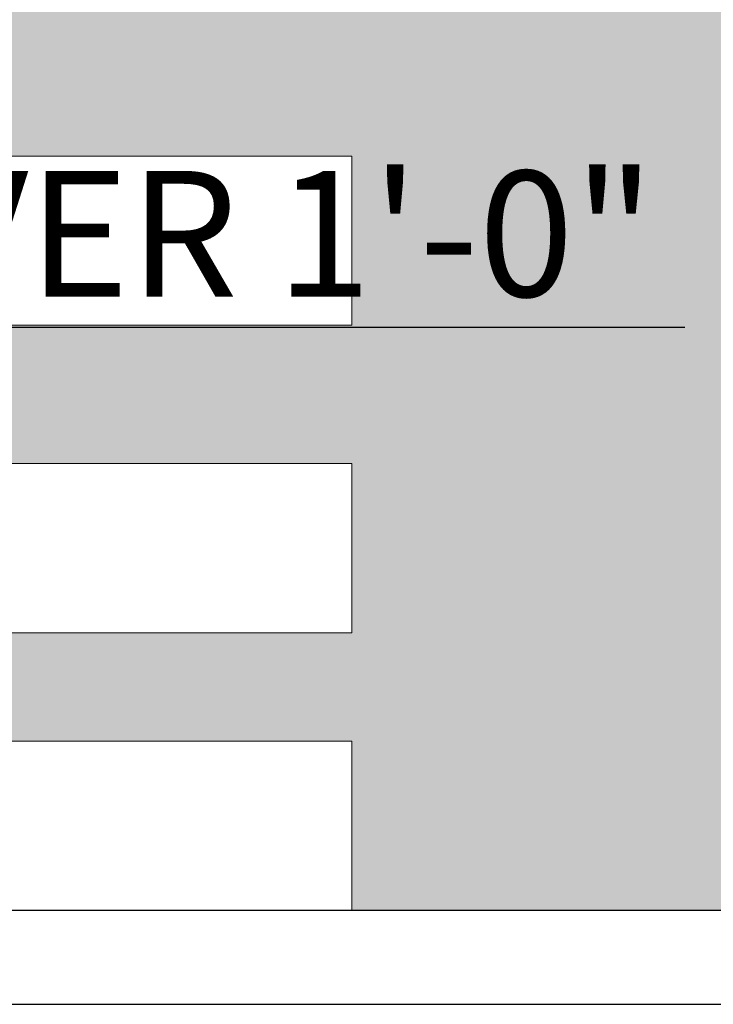
# Model space of a CAD drawing. Units: inches. Extents: x 459864 to 460310, y 324185 to 324787.
# Tile 43 of 112: x 460094 to 460127, y 324195 to 324242. Entities that reach past the tile are written whole.
import ezdxf

# ---------------------------------------------------------------- set-up
doc = ezdxf.new("R2010")
doc.units = ezdxf.units.IN
for name, color, linetype, lineweight in [('A-ANNO-DIMS', 2, 'Continuous', 18), ('C-PROP', 7, 'Continuous', 30), ('L-HRDS', 9, 'Continuous', 18), ('L-SITE-PATT', 252, 'Continuous', 13)]:
    doc.layers.add(name, color=color, linetype=linetype, lineweight=lineweight)
doc.styles.get("Standard").update_dxf_attribs({"font": 'arial.ttf'})
doc.dimstyles.new('ISO-25', dxfattribs={"dimtxt": 6, "dimasz": 2.5, "dimexe": 1.25, "dimexo": 0.625, "dimtad": 1, "dimdec": 1, "dimlunit": 3, "dimtxsty": 'Standard', "dimcen": 2.5, "dimadec": 0, "dimazin": 0, "dimtfac": 1, "dimtdec": 1, "dimtmove": 0, "dimatfit": 3, "dimfxl": 1, "dimarcsym": 0})

# ---------------------------------------------------------------- blocks, each defined once
blk = doc.blocks.new('*D28')
at = {"layer": 'A-ANNO-DIMS', "color": 0, "lineweight": -2, "transparency": 16777216}
for p, q in [((460148.65, 324370.7), (460136.025, 324370.7)), ((460137.275, 324368.2), (460137.275, 324293.2)), ((460148.65, 324290.7), (460136.025, 324290.7)), ((460137.275, 324290.7), (460137.275, 324198.69))]:
    blk.add_line(p, q, dxfattribs=at)
at = {"layer": 'A-ANNO-DIMS', "color": 0, "transparency": 16777216}
for points in [[(460136.858, 324368.2), (460137.692, 324368.2), (460137.275, 324370.7)], [(460136.858, 324293.2), (460137.692, 324293.2), (460137.275, 324290.7)]]:
    blk.add_solid(points, dxfattribs=at)
at = {"layer": 'Defpoints', "color": 0, "transparency": 16777216}
for p in [(460149.275, 324370.7), (460137.275, 324290.7), (460149.275, 324290.7)]:
    blk.add_point(p, dxfattribs=at)
at = {"layer": 'A-ANNO-DIMS', "color": 0, "transparency": 16777216, "insert": (460133.363, 324243.445), "char_height": 6, "attachment_point": 5, "rotation": 90}
blk.add_mtext('QUEEN BED 6\'-8" TYP.', dxfattribs=at)
blk = doc.blocks.new('*D36')
at = {"layer": 'A-ANNO-DIMS', "color": 0, "lineweight": -2, "transparency": 16777216}
for p, q in [((460063.861, 324228.483), (460063.861, 324226.056)), ((460075.876, 324228.483), (460075.876, 324226.056)), ((460066.361, 324227.306), (460073.376, 324227.306)), ((460075.876, 324227.306), (460126.021, 324227.306))]:
    blk.add_line(p, q, dxfattribs=at)
at = {"layer": 'A-ANNO-DIMS', "color": 0, "transparency": 16777216}
for points in [[(460066.361, 324227.722), (460066.361, 324226.889), (460063.861, 324227.306)], [(460073.376, 324227.722), (460073.376, 324226.889), (460075.876, 324227.306)]]:
    blk.add_solid(points, dxfattribs=at)
at = {"layer": 'Defpoints', "color": 0, "transparency": 16777216}
for p in [(460063.861, 324229.108), (460075.876, 324229.108), (460075.876, 324227.306)]:
    blk.add_point(p, dxfattribs=at)
at = {"layer": 'A-ANNO-DIMS', "color": 0, "transparency": 16777216, "insert": (460102.199, 324230.994), "char_height": 6, "attachment_point": 5}
blk.add_mtext('PAVER 1\'-0"', dxfattribs=at)

msp = doc.modelspace()

# ---------------------------------------------------------------- hatches: boundary and pattern name
at = {"layer": 'L-SITE-PATT'}
h = msp.add_hatch(dxfattribs=at)
h.set_pattern_fill('DOTS', color=256)
h.paths.add_polyline_path([(460269.804, 324283.483), (460247.115, 324283.483), (460121.929, 324283.483), (460121.929, 324252.473), (460117.429, 324252.473), (460110.124, 324252.473), (460110.124, 324243.287), (460080.83, 324243.287), (460080.83, 324252.473), (460061.115, 324252.473), (460061.115, 324251.882), (460077.909, 324251.882), (460077.909, 324199.483), (460080.83, 324199.483), (460080.83, 324207.553), (460110.124, 324207.553), (460110.124, 324199.483), (460110.813, 324199.483), (460262.115, 324199.483), (460269.804, 324199.483)], flags=17)
edge = h.paths.add_edge_path(flags=0)
edge.add_ellipse((460222.59, 324263.813), major_axis=(-8.485, 8.485), ratio=1, start_angle=405, end_angle=495, ccw=False)
edge.add_line((460214.821, 324254.66), (460214.832, 324254.666))
edge.add_ellipse((460222.59, 324263.813), major_axis=(-8.485, 8.485), ratio=1, start_angle=405, end_angle=495, ccw=False)
edge.add_line((460210.759, 324261.781), (460210.768, 324261.787))
edge.add_ellipse((460222.59, 324263.813), major_axis=(-8.485, 8.485), ratio=1, start_angle=405, end_angle=495, ccw=False)
edge.add_ellipse((460222.59, 324263.813), major_axis=(-8.485, 8.485), ratio=1, start_angle=392.754, end_angle=405, ccw=False)
edge.add_ellipse((460222.59, 324263.813), major_axis=(-8.485, 8.485), ratio=1, start_angle=380.9347, end_angle=392.754, ccw=False)
edge.add_line((460211.337, 324267.985), (460211.34, 324267.985))
edge.add_ellipse((460222.59, 324263.813), major_axis=(-8.485, 8.485), ratio=1, start_angle=380.9347, end_angle=392.754, ccw=False)
edge.add_ellipse((460222.59, 324263.813), major_axis=(-8.485, 8.485), ratio=1, start_angle=347.9015, end_angle=380.9347, ccw=False)
edge.add_ellipse((460222.59, 324263.813), major_axis=(-8.485, 8.485), ratio=1, start_angle=327.0619, end_angle=347.9015, ccw=False)
edge.add_ellipse((460222.59, 324263.813), major_axis=(-8.485, 8.485), ratio=1, start_angle=278.3246, end_angle=327.0619, ccw=False)
edge.add_line((460225.158, 324275.536), (460225.158, 324275.535))
edge.add_ellipse((460222.59, 324263.813), major_axis=(-8.485, 8.485), ratio=1, start_angle=278.3246, end_angle=327.0619, ccw=False)
edge.add_ellipse((460222.59, 324263.813), major_axis=(-8.485, 8.485), ratio=1, start_angle=260.6436, end_angle=278.3246, ccw=False)
edge.add_ellipse((460222.59, 324263.813), major_axis=(-8.485, 8.485), ratio=1, start_angle=225, end_angle=260.6436, ccw=False)
edge.add_line((460234.509, 324265.243), (460234.501, 324265.239))
edge.add_ellipse((460222.59, 324263.813), major_axis=(-8.485, 8.485), ratio=1, start_angle=225, end_angle=260.6436, ccw=False)
edge.add_ellipse((460222.59, 324263.813), major_axis=(-8.485, 8.485), ratio=1, start_angle=495, end_angle=585, ccw=False)
edge.add_line((460234.437, 324261.861), (460234.424, 324261.858))
edge.add_ellipse((460222.59, 324263.813), major_axis=(-8.485, 8.485), ratio=1, start_angle=495, end_angle=585, ccw=False)
edge.add_line((460227.95, 324253.067), (460227.946, 324253.083))
edge.add_ellipse((460222.59, 324263.813), major_axis=(-8.485, 8.485), ratio=1, start_angle=495, end_angle=585, ccw=False)
edge.add_line((460226.223, 324252.369), (460226.211, 324252.38))
edge.add_ellipse((460222.59, 324263.813), major_axis=(-8.485, 8.485), ratio=1, start_angle=495, end_angle=585, ccw=False)
h.paths.add_polyline_path([(460219.651, 324254.347), (460218.461, 324253.545), (460218.275, 324254.789), (460219.642, 324256.542), (460219.625, 324260.848), (460216.11, 324257.333), (460214.35, 324256.978), (460215.416, 324259.356), (460212.524, 324258.496), (460213.137, 324259.93), (460218.507, 324263.813), (460222.59, 324263.813), (460222.59, 324267.807), (460218.176, 324272.212), (460219.026, 324274.639), (460222.59, 324272.811), (460222.59, 324275.423), (460223.057, 324274.825), (460222.675, 324273.492), (460225.912, 324267.135), (460219.625, 324260.848)], flags=0)
edge = h.paths.add_edge_path(flags=0)
edge.add_ellipse((460194.576, 324264.046), major_axis=(-8.485, 8.485), ratio=1, start_angle=495, end_angle=585, ccw=False)
edge.add_line((460199.936, 324253.3), (460199.932, 324253.316))
edge.add_ellipse((460194.576, 324264.046), major_axis=(-8.485, 8.485), ratio=1, start_angle=495, end_angle=585, ccw=False)
edge.add_line((460198.208, 324252.603), (460198.196, 324252.613))
edge.add_ellipse((460194.576, 324264.046), major_axis=(-8.485, 8.485), ratio=1, start_angle=495, end_angle=585, ccw=False)
edge.add_ellipse((460194.576, 324264.046), major_axis=(-8.485, 8.485), ratio=1, start_angle=405, end_angle=495, ccw=False)
edge.add_line((460186.806, 324254.893), (460186.817, 324254.899))
edge.add_ellipse((460194.576, 324264.046), major_axis=(-8.485, 8.485), ratio=1, start_angle=405, end_angle=495, ccw=False)
edge.add_line((460182.744, 324262.014), (460182.753, 324262.02))
edge.add_ellipse((460194.576, 324264.046), major_axis=(-8.485, 8.485), ratio=1, start_angle=405, end_angle=495, ccw=False)
edge.add_ellipse((460194.576, 324264.046), major_axis=(-8.485, 8.485), ratio=1, start_angle=392.754, end_angle=405, ccw=False)
edge.add_ellipse((460194.576, 324264.046), major_axis=(-8.485, 8.485), ratio=1, start_angle=380.9347, end_angle=392.754, ccw=False)
edge.add_line((460183.323, 324268.218), (460183.326, 324268.218))
edge.add_ellipse((460194.576, 324264.046), major_axis=(-8.485, 8.485), ratio=1, start_angle=380.9347, end_angle=392.754, ccw=False)
edge.add_ellipse((460194.576, 324264.046), major_axis=(-8.485, 8.485), ratio=1, start_angle=347.9015, end_angle=380.9347, ccw=False)
edge.add_ellipse((460194.576, 324264.046), major_axis=(-8.485, 8.485), ratio=1, start_angle=327.0619, end_angle=347.9015, ccw=False)
edge.add_ellipse((460194.576, 324264.046), major_axis=(-8.485, 8.485), ratio=1, start_angle=278.3246, end_angle=327.0619, ccw=False)
edge.add_line((460197.144, 324275.769), (460197.143, 324275.768))
edge.add_ellipse((460194.576, 324264.046), major_axis=(-8.485, 8.485), ratio=1, start_angle=278.3246, end_angle=327.0619, ccw=False)
edge.add_ellipse((460194.576, 324264.046), major_axis=(-8.485, 8.485), ratio=1, start_angle=260.6436, end_angle=278.3246, ccw=False)
edge.add_ellipse((460194.576, 324264.046), major_axis=(-8.485, 8.485), ratio=1, start_angle=225, end_angle=260.6436, ccw=False)
edge.add_line((460206.494, 324265.476), (460206.487, 324265.473))
edge.add_ellipse((460194.576, 324264.046), major_axis=(-8.485, 8.485), ratio=1, start_angle=225, end_angle=260.6436, ccw=False)
edge.add_ellipse((460194.576, 324264.046), major_axis=(-8.485, 8.485), ratio=1, start_angle=495, end_angle=585, ccw=False)
edge.add_line((460206.422, 324262.094), (460206.409, 324262.091))
h.paths.add_polyline_path([(460191.61, 324261.081), (460191.637, 324254.58), (460190.447, 324253.778), (460190.261, 324255.023), (460191.628, 324256.775), (460191.61, 324261.081), (460188.096, 324257.566), (460186.335, 324257.211), (460187.402, 324259.589), (460184.509, 324258.729), (460185.123, 324260.163), (460190.493, 324264.046), (460194.576, 324264.046), (460194.576, 324268.04), (460190.161, 324272.446), (460191.011, 324274.872), (460194.576, 324273.044), (460194.576, 324275.657), (460195.043, 324275.058), (460194.661, 324273.725), (460197.897, 324267.368)], flags=0)
edge = h.paths.add_edge_path(flags=0)
edge.add_ellipse((460252.912, 324263.578), major_axis=(-8.485, 8.485), ratio=1, start_angle=405, end_angle=495, ccw=False)
edge.add_line((460241.081, 324261.545), (460241.089, 324261.551))
edge.add_ellipse((460252.912, 324263.578), major_axis=(-8.485, 8.485), ratio=1, start_angle=405, end_angle=495, ccw=False)
edge.add_ellipse((460252.912, 324263.578), major_axis=(-8.485, 8.485), ratio=1, start_angle=392.754, end_angle=405, ccw=False)
edge.add_ellipse((460252.912, 324263.578), major_axis=(-8.485, 8.485), ratio=1, start_angle=380.9347, end_angle=392.754, ccw=False)
edge.add_line((460241.659, 324267.749), (460241.662, 324267.749))
edge.add_ellipse((460252.912, 324263.578), major_axis=(-8.485, 8.485), ratio=1, start_angle=380.9347, end_angle=392.754, ccw=False)
edge.add_ellipse((460252.912, 324263.578), major_axis=(-8.485, 8.485), ratio=1, start_angle=347.9015, end_angle=380.9347, ccw=False)
edge.add_ellipse((460252.912, 324263.578), major_axis=(-8.485, 8.485), ratio=1, start_angle=327.0619, end_angle=347.9015, ccw=False)
edge.add_ellipse((460252.912, 324263.578), major_axis=(-8.485, 8.485), ratio=1, start_angle=278.3246, end_angle=327.0619, ccw=False)
edge.add_line((460255.48, 324275.3), (460255.479, 324275.299))
edge.add_ellipse((460252.912, 324263.578), major_axis=(-8.485, 8.485), ratio=1, start_angle=278.3246, end_angle=327.0619, ccw=False)
edge.add_ellipse((460252.912, 324263.578), major_axis=(-8.485, 8.485), ratio=1, start_angle=260.6436, end_angle=278.3246, ccw=False)
edge.add_ellipse((460252.912, 324263.578), major_axis=(-8.485, 8.485), ratio=1, start_angle=225, end_angle=260.6436, ccw=False)
edge.add_line((460264.83, 324265.007), (460264.823, 324265.004))
edge.add_ellipse((460252.912, 324263.578), major_axis=(-8.485, 8.485), ratio=1, start_angle=225, end_angle=260.6436, ccw=False)
edge.add_ellipse((460252.912, 324263.578), major_axis=(-8.485, 8.485), ratio=1, start_angle=495, end_angle=585, ccw=False)
edge.add_line((460264.758, 324261.626), (460264.745, 324261.622))
edge.add_ellipse((460252.912, 324263.578), major_axis=(-8.485, 8.485), ratio=1, start_angle=495, end_angle=585, ccw=False)
edge.add_line((460258.272, 324252.832), (460258.268, 324252.848))
edge.add_ellipse((460252.912, 324263.578), major_axis=(-8.485, 8.485), ratio=1, start_angle=495, end_angle=585, ccw=False)
edge.add_line((460256.545, 324252.134), (460256.533, 324252.144))
edge.add_ellipse((460252.912, 324263.578), major_axis=(-8.485, 8.485), ratio=1, start_angle=495, end_angle=585, ccw=False)
edge.add_ellipse((460252.912, 324263.578), major_axis=(-8.485, 8.485), ratio=1, start_angle=405, end_angle=495, ccw=False)
edge.add_line((460245.143, 324254.424), (460245.153, 324254.43))
h.paths.add_polyline_path([(460244.672, 324256.742), (460245.738, 324259.12), (460242.846, 324258.26), (460243.459, 324259.694), (460248.829, 324263.578), (460252.912, 324263.578), (460252.912, 324267.571), (460248.497, 324271.977), (460249.348, 324274.403), (460252.912, 324272.576), (460252.912, 324275.188), (460253.379, 324274.589), (460252.997, 324273.257), (460256.233, 324266.899), (460249.946, 324260.612), (460249.973, 324254.111), (460248.783, 324253.309), (460248.597, 324254.554), (460249.964, 324256.306), (460249.946, 324260.612), (460246.432, 324257.097)], flags=0)
edge = h.paths.add_edge_path(flags=0)
edge.add_ellipse((460167.439, 324262.833), major_axis=(-8.485, 8.485), ratio=1, start_angle=495, end_angle=585, ccw=False)
edge.add_line((460172.799, 324252.087), (460172.795, 324252.103))
edge.add_ellipse((460167.439, 324262.833), major_axis=(-8.485, 8.485), ratio=1, start_angle=495, end_angle=585, ccw=False)
edge.add_line((460171.071, 324251.389), (460171.059, 324251.399))
edge.add_ellipse((460167.439, 324262.833), major_axis=(-8.485, 8.485), ratio=1, start_angle=495, end_angle=585, ccw=False)
edge.add_ellipse((460167.439, 324262.833), major_axis=(-8.485, 8.485), ratio=1, start_angle=405, end_angle=495, ccw=False)
edge.add_line((460159.669, 324253.679), (460159.68, 324253.685))
edge.add_ellipse((460167.439, 324262.833), major_axis=(-8.485, 8.485), ratio=1, start_angle=405, end_angle=495, ccw=False)
edge.add_line((460155.607, 324260.8), (460155.616, 324260.806))
edge.add_ellipse((460167.439, 324262.833), major_axis=(-8.485, 8.485), ratio=1, start_angle=405, end_angle=495, ccw=False)
edge.add_ellipse((460167.439, 324262.833), major_axis=(-8.485, 8.485), ratio=1, start_angle=392.754, end_angle=405, ccw=False)
edge.add_ellipse((460167.439, 324262.833), major_axis=(-8.485, 8.485), ratio=1, start_angle=380.9347, end_angle=392.754, ccw=False)
edge.add_line((460156.185, 324267.005), (460156.189, 324267.005))
edge.add_ellipse((460167.439, 324262.833), major_axis=(-8.485, 8.485), ratio=1, start_angle=380.9347, end_angle=392.754, ccw=False)
edge.add_ellipse((460167.439, 324262.833), major_axis=(-8.485, 8.485), ratio=1, start_angle=347.9015, end_angle=380.9347, ccw=False)
edge.add_ellipse((460167.439, 324262.833), major_axis=(-8.485, 8.485), ratio=1, start_angle=327.0619, end_angle=347.9015, ccw=False)
edge.add_ellipse((460167.439, 324262.833), major_axis=(-8.485, 8.485), ratio=1, start_angle=278.3246, end_angle=327.0619, ccw=False)
edge.add_line((460170.007, 324274.556), (460170.006, 324274.554))
edge.add_ellipse((460167.439, 324262.833), major_axis=(-8.485, 8.485), ratio=1, start_angle=278.3246, end_angle=327.0619, ccw=False)
edge.add_ellipse((460167.439, 324262.833), major_axis=(-8.485, 8.485), ratio=1, start_angle=260.6436, end_angle=278.3246, ccw=False)
edge.add_ellipse((460167.439, 324262.833), major_axis=(-8.485, 8.485), ratio=1, start_angle=225, end_angle=260.6436, ccw=False)
edge.add_line((460179.357, 324264.262), (460179.35, 324264.259))
edge.add_ellipse((460167.439, 324262.833), major_axis=(-8.485, 8.485), ratio=1, start_angle=225, end_angle=260.6436, ccw=False)
edge.add_ellipse((460167.439, 324262.833), major_axis=(-8.485, 8.485), ratio=1, start_angle=495, end_angle=585, ccw=False)
edge.add_line((460179.285, 324260.881), (460179.272, 324260.877))
h.paths.add_polyline_path([(460164.473, 324259.867), (460164.5, 324253.366), (460163.31, 324252.565), (460163.124, 324253.809), (460164.491, 324255.561), (460164.473, 324259.867), (460160.958, 324256.353), (460159.198, 324255.998), (460160.265, 324258.375), (460157.372, 324257.515), (460157.986, 324258.949), (460163.356, 324262.833), (460167.439, 324262.833), (460167.439, 324266.826), (460163.024, 324271.232), (460163.874, 324273.659), (460167.439, 324271.831), (460167.439, 324274.443), (460167.905, 324273.844), (460167.524, 324272.512), (460170.76, 324266.154)], flags=0)
edge = h.paths.add_edge_path(flags=0)
edge.add_ellipse((460140.758, 324262.37), major_axis=(-8.485, 8.485), ratio=1, start_angle=495, end_angle=585, ccw=False)
edge.add_line((460146.118, 324251.624), (460146.114, 324251.639))
edge.add_ellipse((460140.758, 324262.37), major_axis=(-8.485, 8.485), ratio=1, start_angle=495, end_angle=585, ccw=False)
edge.add_line((460144.391, 324250.926), (460144.379, 324250.936))
edge.add_ellipse((460140.758, 324262.37), major_axis=(-8.485, 8.485), ratio=1, start_angle=495, end_angle=585, ccw=False)
edge.add_ellipse((460140.758, 324262.37), major_axis=(-8.485, 8.485), ratio=1, start_angle=405, end_angle=495, ccw=False)
edge.add_line((460132.989, 324253.216), (460132.999, 324253.222))
edge.add_ellipse((460140.758, 324262.37), major_axis=(-8.485, 8.485), ratio=1, start_angle=405, end_angle=495, ccw=False)
edge.add_line((460128.927, 324260.337), (460128.935, 324260.343))
edge.add_ellipse((460140.758, 324262.37), major_axis=(-8.485, 8.485), ratio=1, start_angle=405, end_angle=495, ccw=False)
edge.add_ellipse((460140.758, 324262.37), major_axis=(-8.485, 8.485), ratio=1, start_angle=392.754, end_angle=405, ccw=False)
edge.add_ellipse((460140.758, 324262.37), major_axis=(-8.485, 8.485), ratio=1, start_angle=380.9347, end_angle=392.754, ccw=False)
edge.add_line((460129.505, 324266.541), (460129.508, 324266.541))
edge.add_ellipse((460140.758, 324262.37), major_axis=(-8.485, 8.485), ratio=1, start_angle=380.9347, end_angle=392.754, ccw=False)
edge.add_ellipse((460140.758, 324262.37), major_axis=(-8.485, 8.485), ratio=1, start_angle=347.9015, end_angle=380.9347, ccw=False)
edge.add_ellipse((460140.758, 324262.37), major_axis=(-8.485, 8.485), ratio=1, start_angle=327.0619, end_angle=347.9015, ccw=False)
edge.add_ellipse((460140.758, 324262.37), major_axis=(-8.485, 8.485), ratio=1, start_angle=278.3246, end_angle=327.0619, ccw=False)
edge.add_line((460143.326, 324274.092), (460143.325, 324274.091))
edge.add_ellipse((460140.758, 324262.37), major_axis=(-8.485, 8.485), ratio=1, start_angle=278.3246, end_angle=327.0619, ccw=False)
edge.add_ellipse((460140.758, 324262.37), major_axis=(-8.485, 8.485), ratio=1, start_angle=260.6436, end_angle=278.3246, ccw=False)
edge.add_ellipse((460140.758, 324262.37), major_axis=(-8.485, 8.485), ratio=1, start_angle=225, end_angle=260.6436, ccw=False)
edge.add_line((460152.677, 324263.799), (460152.669, 324263.796))
edge.add_ellipse((460140.758, 324262.37), major_axis=(-8.485, 8.485), ratio=1, start_angle=225, end_angle=260.6436, ccw=False)
edge.add_ellipse((460140.758, 324262.37), major_axis=(-8.485, 8.485), ratio=1, start_angle=495, end_angle=585, ccw=False)
edge.add_line((460152.604, 324260.418), (460152.592, 324260.414))
h.paths.add_polyline_path([(460137.792, 324259.404), (460137.819, 324252.903), (460136.629, 324252.101), (460136.443, 324253.346), (460137.81, 324255.098), (460137.792, 324259.404), (460134.278, 324255.889), (460132.518, 324255.534), (460133.584, 324257.912), (460130.692, 324257.052), (460131.305, 324258.486), (460136.675, 324262.37), (460140.758, 324262.37), (460140.758, 324266.363), (460136.343, 324270.769), (460137.194, 324273.195), (460140.758, 324271.367), (460140.758, 324273.98), (460141.225, 324273.381), (460140.843, 324272.049), (460144.079, 324265.691)], flags=0)
h.paths.add_polyline_path([(460110.124, 324227.414), (460080.83, 324227.414), (460080.83, 324235.484), (460110.124, 324235.484)], flags=16)
h.paths.add_polyline_path([(460110.124, 324220.797), (460110.124, 324212.727), (460080.83, 324212.727), (460080.83, 324220.797)], flags=16)
h.paths.add_polyline_path([(460269.804, 324283.483), (460247.115, 324283.483), (460121.929, 324283.483), (460121.929, 324252.473), (460117.429, 324252.473), (460110.124, 324252.473), (460110.124, 324243.287), (460080.83, 324243.287), (460080.83, 324252.473), (460061.115, 324252.473), (460061.115, 324251.882), (460077.909, 324251.882), (460077.909, 324199.483), (460080.83, 324199.483), (460080.83, 324207.553), (460110.124, 324207.553), (460110.124, 324199.483), (460262.115, 324199.483), (460269.804, 324199.483)], flags=17)
h.paths.add_polyline_path([(460219.651, 324254.347), (460218.461, 324253.545), (460218.275, 324254.789), (460219.642, 324256.542), (460219.625, 324260.848), (460216.11, 324257.333), (460214.35, 324256.978), (460215.416, 324259.356), (460212.524, 324258.496), (460213.137, 324259.93), (460218.507, 324263.813), (460222.59, 324263.813), (460220.18, 324266.223), (460215.461, 324265.308), (460211.835, 324266.137), (460216.247, 324267.985), (460218.418, 324267.985), (460222.59, 324263.813), (460222.59, 324267.807), (460218.176, 324272.212), (460219.026, 324274.639), (460222.59, 324272.811), (460222.59, 324275.423), (460223.057, 324274.825), (460222.675, 324273.492), (460225.912, 324267.135), (460222.59, 324263.813), (460231.383, 324263.813), (460228.485, 324262.488), (460224.425, 324261.978), (460228.68, 324257.724), (460228.966, 324254.791), (460227.142, 324256.537), (460227.542, 324254.819), (460227.333, 324253.614), (460222.59, 324259.985), (460222.59, 324255.497), (460221.377, 324256.541), (460220.576, 324261.799), (460219.625, 324260.848)], flags=0)
h.paths.add_polyline_path([(460199.127, 324256.77), (460199.528, 324255.052), (460199.319, 324253.848), (460194.576, 324260.218), (460194.576, 324255.73), (460193.363, 324256.774), (460192.561, 324262.032), (460191.61, 324261.081), (460191.637, 324254.58), (460190.447, 324253.778), (460190.261, 324255.023), (460191.628, 324256.775), (460191.61, 324261.081), (460188.096, 324257.566), (460186.335, 324257.211), (460187.402, 324259.589), (460184.509, 324258.729), (460185.123, 324260.163), (460190.493, 324264.046), (460194.576, 324264.046), (460192.166, 324266.456), (460187.446, 324265.541), (460183.82, 324266.37), (460188.232, 324268.218), (460190.404, 324268.218), (460194.576, 324264.046), (460194.576, 324268.04), (460190.161, 324272.446), (460191.011, 324274.872), (460194.576, 324273.044), (460194.576, 324275.657), (460195.043, 324275.058), (460194.661, 324273.725), (460197.897, 324267.368), (460194.576, 324264.046), (460203.368, 324264.046), (460200.47, 324262.721), (460196.411, 324262.212), (460200.665, 324257.957), (460200.951, 324255.024)], flags=0)
h.paths.add_polyline_path([(460244.672, 324256.742), (460245.738, 324259.12), (460242.846, 324258.26), (460243.459, 324259.694), (460248.829, 324263.578), (460252.912, 324263.578), (460250.502, 324265.987), (460245.783, 324265.072), (460242.156, 324265.901), (460246.568, 324267.749), (460248.74, 324267.749), (460252.912, 324263.578), (460252.912, 324267.571), (460248.497, 324271.977), (460249.348, 324274.403), (460252.912, 324272.576), (460252.912, 324275.188), (460253.379, 324274.589), (460252.997, 324273.257), (460256.233, 324266.899), (460252.912, 324263.578), (460261.705, 324263.578), (460258.806, 324262.252), (460254.747, 324261.743), (460259.002, 324257.488), (460259.288, 324254.555), (460257.463, 324256.301), (460257.864, 324254.583), (460257.655, 324253.379), (460252.912, 324259.749), (460252.912, 324255.261), (460251.699, 324256.305), (460250.897, 324261.563), (460249.946, 324260.612), (460249.973, 324254.111), (460248.783, 324253.309), (460248.597, 324254.554), (460249.964, 324256.306), (460249.946, 324260.612), (460246.432, 324257.097)], flags=0)
h.paths.add_polyline_path([(460173.528, 324256.743), (460173.814, 324253.811), (460171.99, 324255.556), (460172.39, 324253.838), (460172.182, 324252.634), (460167.439, 324259.004), (460167.439, 324254.516), (460166.226, 324255.56), (460165.424, 324260.818), (460164.473, 324259.867), (460164.5, 324253.366), (460163.31, 324252.565), (460163.124, 324253.809), (460164.491, 324255.561), (460164.473, 324259.867), (460160.958, 324256.353), (460159.198, 324255.998), (460160.265, 324258.375), (460157.372, 324257.515), (460157.986, 324258.949), (460163.356, 324262.833), (460167.439, 324262.833), (460165.029, 324265.243), (460160.309, 324264.327), (460156.683, 324265.156), (460161.095, 324267.005), (460163.267, 324267.005), (460167.439, 324262.833), (460167.439, 324266.826), (460163.024, 324271.232), (460163.874, 324273.659), (460167.439, 324271.831), (460167.439, 324274.443), (460167.905, 324273.844), (460167.524, 324272.512), (460170.76, 324266.154), (460167.439, 324262.833), (460176.231, 324262.833), (460173.333, 324261.507), (460169.274, 324260.998)], flags=0)
h.paths.add_polyline_path([(460146.848, 324256.28), (460147.134, 324253.347), (460145.31, 324255.093), (460145.71, 324253.375), (460145.501, 324252.171), (460140.758, 324258.541), (460140.758, 324254.053), (460139.545, 324255.097), (460138.744, 324260.355), (460137.792, 324259.404), (460137.819, 324252.903), (460136.629, 324252.101), (460136.443, 324253.346), (460137.81, 324255.098), (460137.792, 324259.404), (460134.278, 324255.889), (460132.518, 324255.534), (460133.584, 324257.912), (460130.692, 324257.052), (460131.305, 324258.486), (460136.675, 324262.37), (460140.758, 324262.37), (460138.348, 324264.779), (460133.629, 324263.864), (460130.002, 324264.693), (460134.414, 324266.541), (460136.586, 324266.541), (460140.758, 324262.37), (460140.758, 324266.363), (460136.343, 324270.769), (460137.194, 324273.195), (460140.758, 324271.367), (460140.758, 324273.98), (460141.225, 324273.381), (460140.843, 324272.049), (460144.079, 324265.691), (460140.758, 324262.37), (460149.551, 324262.37), (460146.653, 324261.044), (460142.593, 324260.535)], flags=0)
edge = h.paths.add_edge_path()
edge.add_line((460269.804, 324272.549), (460260.881, 324272.549))
edge.add_ellipse((460252.912, 324263.578), major_axis=(-8.485, 8.485), ratio=1, start_angle=260.6436, end_angle=273.3846, ccw=False)
edge.add_line((460262.283, 324271.092), (460262.261, 324271.091))
edge.add_ellipse((460252.912, 324263.578), major_axis=(-8.485, 8.485), ratio=1, start_angle=260.6436, end_angle=273.3846, ccw=False)
edge.add_ellipse((460252.912, 324263.578), major_axis=(-8.485, 8.485), ratio=1, start_angle=225, end_angle=260.6436, ccw=False)
edge.add_line((460263.609, 324269.063), (460263.572, 324269.058))
edge.add_ellipse((460252.912, 324263.578), major_axis=(-8.485, 8.485), ratio=1, start_angle=225, end_angle=260.6436, ccw=False)
edge.add_line((460264.615, 324266.306), (460264.585, 324266.305))
edge.add_ellipse((460252.912, 324263.578), major_axis=(-8.485, 8.485), ratio=1, start_angle=225, end_angle=260.6436, ccw=False)
edge.add_line((460264.83, 324265.007), (460264.823, 324265.004))
edge.add_ellipse((460252.912, 324263.578), major_axis=(-8.485, 8.485), ratio=1, start_angle=225, end_angle=260.6436, ccw=False)
edge.add_ellipse((460252.912, 324263.578), major_axis=(-8.485, 8.485), ratio=1, start_angle=495, end_angle=585, ccw=False)
edge.add_line((460264.758, 324261.626), (460264.745, 324261.622))
edge.add_ellipse((460252.912, 324263.578), major_axis=(-8.485, 8.485), ratio=1, start_angle=495, end_angle=585, ccw=False)
edge.add_line((460263.442, 324257.739), (460263.389, 324257.779))
edge.add_ellipse((460252.912, 324263.578), major_axis=(-8.485, 8.485), ratio=1, start_angle=495, end_angle=585, ccw=False)
edge.add_line((460258.128, 324252.744), (460258.102, 324252.779))
edge.add_ellipse((460252.912, 324263.578), major_axis=(-8.485, 8.485), ratio=1, start_angle=495, end_angle=585, ccw=False)
edge.add_line((460256.545, 324252.134), (460256.533, 324252.144))
edge.add_ellipse((460252.912, 324263.578), major_axis=(-8.485, 8.485), ratio=1, start_angle=495, end_angle=585, ccw=False)
edge.add_ellipse((460252.912, 324263.578), major_axis=(-8.485, 8.485), ratio=1, start_angle=405, end_angle=495, ccw=False)
edge.add_line((460250.594, 324251.78), (460250.605, 324251.82))
edge.add_ellipse((460252.912, 324263.578), major_axis=(-8.485, 8.485), ratio=1, start_angle=405, end_angle=495, ccw=False)
edge.add_line((460245.143, 324254.424), (460245.153, 324254.43))
edge.add_ellipse((460252.912, 324263.578), major_axis=(-8.485, 8.485), ratio=1, start_angle=405, end_angle=495, ccw=False)
edge.add_line((460243.525, 324256.059), (460243.56, 324256.091))
edge.add_ellipse((460252.912, 324263.578), major_axis=(-8.485, 8.485), ratio=1, start_angle=405, end_angle=495, ccw=False)
edge.add_line((460241.44, 324259.893), (460241.522, 324259.896))
edge.add_ellipse((460252.912, 324263.578), major_axis=(-8.485, 8.485), ratio=1, start_angle=405, end_angle=495, ccw=False)
edge.add_line((460241.081, 324261.545), (460241.089, 324261.551))
edge.add_ellipse((460252.912, 324263.578), major_axis=(-8.485, 8.485), ratio=1, start_angle=405, end_angle=495, ccw=False)
edge.add_ellipse((460252.912, 324263.578), major_axis=(-8.485, 8.485), ratio=1, start_angle=392.754, end_angle=405, ccw=False)
edge.add_line((460241.05, 324265.438), (460241.063, 324265.443))
edge.add_ellipse((460252.912, 324263.578), major_axis=(-8.485, 8.485), ratio=1, start_angle=392.754, end_angle=405, ccw=False)
edge.add_ellipse((460252.912, 324263.578), major_axis=(-8.485, 8.485), ratio=1, start_angle=380.9347, end_angle=392.754, ccw=False)
edge.add_line((460241.452, 324267.176), (460241.469, 324267.171))
edge.add_ellipse((460252.912, 324263.578), major_axis=(-8.485, 8.485), ratio=1, start_angle=380.9347, end_angle=392.754, ccw=False)
edge.add_line((460241.659, 324267.749), (460241.662, 324267.749))
edge.add_ellipse((460252.912, 324263.578), major_axis=(-8.485, 8.485), ratio=1, start_angle=380.9347, end_angle=392.754, ccw=False)
edge.add_ellipse((460252.912, 324263.578), major_axis=(-8.485, 8.485), ratio=1, start_angle=356.6154, end_angle=380.9347, ccw=False)
edge.add_line((460244.88, 324272.488), (460244.713, 324272.549))
edge.add_line((460244.713, 324272.549), (460230.817, 324272.549))
edge.add_ellipse((460222.59, 324263.813), major_axis=(-8.485, 8.485), ratio=1, start_angle=260.6436, end_angle=271.7178, ccw=False)
edge.add_ellipse((460222.59, 324263.813), major_axis=(-8.485, 8.485), ratio=1, start_angle=225, end_angle=260.6436, ccw=False)
edge.add_line((460233.287, 324269.299), (460233.25, 324269.294))
edge.add_ellipse((460222.59, 324263.813), major_axis=(-8.485, 8.485), ratio=1, start_angle=225, end_angle=260.6436, ccw=False)
edge.add_line((460234.294, 324266.541), (460234.264, 324266.541))
edge.add_ellipse((460222.59, 324263.813), major_axis=(-8.485, 8.485), ratio=1, start_angle=225, end_angle=260.6436, ccw=False)
edge.add_line((460234.509, 324265.243), (460234.501, 324265.239))
edge.add_ellipse((460222.59, 324263.813), major_axis=(-8.485, 8.485), ratio=1, start_angle=225, end_angle=260.6436, ccw=False)
edge.add_ellipse((460222.59, 324263.813), major_axis=(-8.485, 8.485), ratio=1, start_angle=495, end_angle=585, ccw=False)
edge.add_line((460234.437, 324261.861), (460234.424, 324261.858))
edge.add_ellipse((460222.59, 324263.813), major_axis=(-8.485, 8.485), ratio=1, start_angle=495, end_angle=585, ccw=False)
edge.add_line((460233.121, 324257.975), (460233.068, 324258.015))
edge.add_ellipse((460222.59, 324263.813), major_axis=(-8.485, 8.485), ratio=1, start_angle=495, end_angle=585, ccw=False)
edge.add_line((460227.806, 324252.979), (460227.78, 324253.014))
edge.add_ellipse((460222.59, 324263.813), major_axis=(-8.485, 8.485), ratio=1, start_angle=495, end_angle=585, ccw=False)
edge.add_line((460226.223, 324252.369), (460226.211, 324252.38))
edge.add_ellipse((460222.59, 324263.813), major_axis=(-8.485, 8.485), ratio=1, start_angle=495, end_angle=585, ccw=False)
edge.add_ellipse((460222.59, 324263.813), major_axis=(-8.485, 8.485), ratio=1, start_angle=405, end_angle=495, ccw=False)
edge.add_line((460220.272, 324252.016), (460220.283, 324252.055))
edge.add_ellipse((460222.59, 324263.813), major_axis=(-8.485, 8.485), ratio=1, start_angle=405, end_angle=495, ccw=False)
edge.add_line((460214.821, 324254.66), (460214.832, 324254.666))
edge.add_ellipse((460222.59, 324263.813), major_axis=(-8.485, 8.485), ratio=1, start_angle=405, end_angle=495, ccw=False)
edge.add_line((460213.203, 324256.295), (460213.239, 324256.327))
edge.add_ellipse((460222.59, 324263.813), major_axis=(-8.485, 8.485), ratio=1, start_angle=405, end_angle=495, ccw=False)
edge.add_line((460211.118, 324260.128), (460211.201, 324260.131))
edge.add_ellipse((460222.59, 324263.813), major_axis=(-8.485, 8.485), ratio=1, start_angle=405, end_angle=495, ccw=False)
edge.add_line((460210.759, 324261.781), (460210.768, 324261.787))
edge.add_ellipse((460222.59, 324263.813), major_axis=(-8.485, 8.485), ratio=1, start_angle=405, end_angle=495, ccw=False)
edge.add_ellipse((460222.59, 324263.813), major_axis=(-8.485, 8.485), ratio=1, start_angle=392.754, end_angle=405, ccw=False)
edge.add_line((460210.729, 324265.673), (460210.741, 324265.678))
edge.add_ellipse((460222.59, 324263.813), major_axis=(-8.485, 8.485), ratio=1, start_angle=392.754, end_angle=405, ccw=False)
edge.add_ellipse((460222.59, 324263.813), major_axis=(-8.485, 8.485), ratio=1, start_angle=380.9347, end_angle=392.754, ccw=False)
edge.add_line((460211.13, 324267.412), (460211.147, 324267.407))
edge.add_ellipse((460222.59, 324263.813), major_axis=(-8.485, 8.485), ratio=1, start_angle=380.9347, end_angle=392.754, ccw=False)
edge.add_line((460211.337, 324267.985), (460211.34, 324267.985))
edge.add_ellipse((460222.59, 324263.813), major_axis=(-8.485, 8.485), ratio=1, start_angle=380.9347, end_angle=392.754, ccw=False)
edge.add_ellipse((460222.59, 324263.813), major_axis=(-8.485, 8.485), ratio=1, start_angle=358.2822, end_angle=380.9347, ccw=False)
edge.add_line((460213.705, 324271.902), (460213.709, 324271.869))
edge.add_ellipse((460222.59, 324263.813), major_axis=(-8.485, 8.485), ratio=1, start_angle=358.2822, end_angle=380.9347, ccw=False)
edge.add_line((460214.363, 324272.549), (460203.078, 324272.549))
edge.add_line((460203.078, 324272.549), (460203.06, 324272.531))
edge.add_ellipse((460194.576, 324264.046), major_axis=(-8.485, 8.485), ratio=1, start_angle=260.6436, end_angle=270.1168, ccw=False)
edge.add_line((460203.957, 324271.561), (460203.921, 324271.56))
edge.add_ellipse((460194.576, 324264.046), major_axis=(-8.485, 8.485), ratio=1, start_angle=260.6436, end_angle=270.1168, ccw=False)
edge.add_ellipse((460194.576, 324264.046), major_axis=(-8.485, 8.485), ratio=1, start_angle=225, end_angle=260.6436, ccw=False)
edge.add_line((460205.272, 324269.532), (460205.235, 324269.527))
edge.add_ellipse((460194.576, 324264.046), major_axis=(-8.485, 8.485), ratio=1, start_angle=225, end_angle=260.6436, ccw=False)
edge.add_line((460206.279, 324266.774), (460206.249, 324266.774))
edge.add_ellipse((460194.576, 324264.046), major_axis=(-8.485, 8.485), ratio=1, start_angle=225, end_angle=260.6436, ccw=False)
edge.add_line((460206.494, 324265.476), (460206.487, 324265.473))
edge.add_ellipse((460194.576, 324264.046), major_axis=(-8.485, 8.485), ratio=1, start_angle=225, end_angle=260.6436, ccw=False)
edge.add_ellipse((460194.576, 324264.046), major_axis=(-8.485, 8.485), ratio=1, start_angle=495, end_angle=585, ccw=False)
edge.add_line((460206.422, 324262.094), (460206.409, 324262.091))
edge.add_ellipse((460194.576, 324264.046), major_axis=(-8.485, 8.485), ratio=1, start_angle=495, end_angle=585, ccw=False)
edge.add_line((460205.106, 324258.208), (460205.053, 324258.248))
edge.add_ellipse((460194.576, 324264.046), major_axis=(-8.485, 8.485), ratio=1, start_angle=495, end_angle=585, ccw=False)
edge.add_line((460199.792, 324253.212), (460199.766, 324253.248))
edge.add_ellipse((460194.576, 324264.046), major_axis=(-8.485, 8.485), ratio=1, start_angle=495, end_angle=585, ccw=False)
edge.add_line((460198.208, 324252.603), (460198.196, 324252.613))
edge.add_ellipse((460194.576, 324264.046), major_axis=(-8.485, 8.485), ratio=1, start_angle=495, end_angle=585, ccw=False)
edge.add_ellipse((460194.576, 324264.046), major_axis=(-8.485, 8.485), ratio=1, start_angle=405, end_angle=495, ccw=False)
edge.add_line((460192.258, 324252.249), (460192.268, 324252.289))
edge.add_ellipse((460194.576, 324264.046), major_axis=(-8.485, 8.485), ratio=1, start_angle=405, end_angle=495, ccw=False)
edge.add_line((460186.806, 324254.893), (460186.817, 324254.899))
edge.add_ellipse((460194.576, 324264.046), major_axis=(-8.485, 8.485), ratio=1, start_angle=405, end_angle=495, ccw=False)
edge.add_line((460185.188, 324256.528), (460185.224, 324256.56))
edge.add_ellipse((460194.576, 324264.046), major_axis=(-8.485, 8.485), ratio=1, start_angle=405, end_angle=495, ccw=False)
edge.add_line((460183.104, 324260.362), (460183.186, 324260.365))
edge.add_ellipse((460194.576, 324264.046), major_axis=(-8.485, 8.485), ratio=1, start_angle=405, end_angle=495, ccw=False)
edge.add_line((460182.744, 324262.014), (460182.753, 324262.02))
edge.add_ellipse((460194.576, 324264.046), major_axis=(-8.485, 8.485), ratio=1, start_angle=405, end_angle=495, ccw=False)
edge.add_ellipse((460194.576, 324264.046), major_axis=(-8.485, 8.485), ratio=1, start_angle=392.754, end_angle=405, ccw=False)
edge.add_line((460182.714, 324265.906), (460182.726, 324265.912))
edge.add_ellipse((460194.576, 324264.046), major_axis=(-8.485, 8.485), ratio=1, start_angle=392.754, end_angle=405, ccw=False)
edge.add_ellipse((460194.576, 324264.046), major_axis=(-8.485, 8.485), ratio=1, start_angle=380.9347, end_angle=392.754, ccw=False)
edge.add_line((460183.116, 324267.645), (460183.133, 324267.64))
edge.add_ellipse((460194.576, 324264.046), major_axis=(-8.485, 8.485), ratio=1, start_angle=380.9347, end_angle=392.754, ccw=False)
edge.add_line((460183.323, 324268.218), (460183.326, 324268.218))
edge.add_ellipse((460194.576, 324264.046), major_axis=(-8.485, 8.485), ratio=1, start_angle=380.9347, end_angle=392.754, ccw=False)
edge.add_ellipse((460194.576, 324264.046), major_axis=(-8.485, 8.485), ratio=1, start_angle=359.8832, end_angle=380.9347, ccw=False)
edge.add_line((460184.491, 324270.611), (460184.553, 324270.611))
edge.add_ellipse((460194.576, 324264.046), major_axis=(-8.485, 8.485), ratio=1, start_angle=359.8832, end_angle=380.9347, ccw=False)
edge.add_line((460185.346, 324271.76), (460185.379, 324271.728))
edge.add_ellipse((460194.576, 324264.046), major_axis=(-8.485, 8.485), ratio=1, start_angle=359.8832, end_angle=380.9347, ccw=False)
edge.add_line((460185.697, 324272.086), (460185.633, 324272.549))
edge.add_line((460185.633, 324272.549), (460174.683, 324272.549))
edge.add_line((460174.683, 324272.549), (460174.606, 324272.457))
edge.add_ellipse((460167.439, 324262.833), major_axis=(-8.485, 8.485), ratio=1, start_angle=260.6436, end_angle=278.3246, ccw=False)
edge.add_ellipse((460167.439, 324262.833), major_axis=(-8.485, 8.485), ratio=1, start_angle=225, end_angle=260.6436, ccw=False)
edge.add_line((460178.135, 324268.318), (460178.098, 324268.313))
edge.add_ellipse((460167.439, 324262.833), major_axis=(-8.485, 8.485), ratio=1, start_angle=225, end_angle=260.6436, ccw=False)
edge.add_line((460179.142, 324265.561), (460179.112, 324265.56))
edge.add_ellipse((460167.439, 324262.833), major_axis=(-8.485, 8.485), ratio=1, start_angle=225, end_angle=260.6436, ccw=False)
edge.add_line((460179.357, 324264.262), (460179.35, 324264.259))
edge.add_ellipse((460167.439, 324262.833), major_axis=(-8.485, 8.485), ratio=1, start_angle=225, end_angle=260.6436, ccw=False)
edge.add_ellipse((460167.439, 324262.833), major_axis=(-8.485, 8.485), ratio=1, start_angle=495, end_angle=585, ccw=False)
edge.add_line((460179.285, 324260.881), (460179.272, 324260.877))
edge.add_ellipse((460167.439, 324262.833), major_axis=(-8.485, 8.485), ratio=1, start_angle=495, end_angle=585, ccw=False)
edge.add_line((460177.969, 324256.994), (460177.916, 324257.034))
edge.add_ellipse((460167.439, 324262.833), major_axis=(-8.485, 8.485), ratio=1, start_angle=495, end_angle=585, ccw=False)
edge.add_line((460172.655, 324251.999), (460172.629, 324252.034))
edge.add_ellipse((460167.439, 324262.833), major_axis=(-8.485, 8.485), ratio=1, start_angle=495, end_angle=585, ccw=False)
edge.add_line((460171.071, 324251.389), (460171.059, 324251.399))
edge.add_ellipse((460167.439, 324262.833), major_axis=(-8.485, 8.485), ratio=1, start_angle=495, end_angle=585, ccw=False)
edge.add_ellipse((460167.439, 324262.833), major_axis=(-8.485, 8.485), ratio=1, start_angle=405, end_angle=495, ccw=False)
edge.add_line((460165.121, 324251.036), (460165.131, 324251.075))
edge.add_ellipse((460167.439, 324262.833), major_axis=(-8.485, 8.485), ratio=1, start_angle=405, end_angle=495, ccw=False)
edge.add_line((460159.669, 324253.679), (460159.68, 324253.685))
edge.add_ellipse((460167.439, 324262.833), major_axis=(-8.485, 8.485), ratio=1, start_angle=405, end_angle=495, ccw=False)
edge.add_line((460158.051, 324255.314), (460158.087, 324255.347))
edge.add_ellipse((460167.439, 324262.833), major_axis=(-8.485, 8.485), ratio=1, start_angle=405, end_angle=495, ccw=False)
edge.add_line((460155.967, 324259.148), (460156.049, 324259.151))
edge.add_ellipse((460167.439, 324262.833), major_axis=(-8.485, 8.485), ratio=1, start_angle=405, end_angle=495, ccw=False)
edge.add_line((460155.607, 324260.8), (460155.616, 324260.806))
edge.add_ellipse((460167.439, 324262.833), major_axis=(-8.485, 8.485), ratio=1, start_angle=405, end_angle=495, ccw=False)
edge.add_ellipse((460167.439, 324262.833), major_axis=(-8.485, 8.485), ratio=1, start_angle=392.754, end_angle=405, ccw=False)
edge.add_line((460155.577, 324264.693), (460155.589, 324264.698))
edge.add_ellipse((460167.439, 324262.833), major_axis=(-8.485, 8.485), ratio=1, start_angle=392.754, end_angle=405, ccw=False)
edge.add_ellipse((460167.439, 324262.833), major_axis=(-8.485, 8.485), ratio=1, start_angle=380.9347, end_angle=392.754, ccw=False)
edge.add_line((460155.979, 324266.432), (460155.996, 324266.426))
edge.add_ellipse((460167.439, 324262.833), major_axis=(-8.485, 8.485), ratio=1, start_angle=380.9347, end_angle=392.754, ccw=False)
edge.add_line((460156.185, 324267.005), (460156.189, 324267.005))
edge.add_ellipse((460167.439, 324262.833), major_axis=(-8.485, 8.485), ratio=1, start_angle=380.9347, end_angle=392.754, ccw=False)
edge.add_ellipse((460167.439, 324262.833), major_axis=(-8.485, 8.485), ratio=1, start_angle=350.9345, end_angle=380.9347, ccw=False)
edge.add_line((460157.363, 324269.397), (460157.414, 324269.397))
edge.add_ellipse((460167.439, 324262.833), major_axis=(-8.485, 8.485), ratio=1, start_angle=350.9345, end_angle=380.9347, ccw=False)
edge.add_line((460158.221, 324270.535), (460158.236, 324270.519))
edge.add_ellipse((460167.439, 324262.833), major_axis=(-8.485, 8.485), ratio=1, start_angle=350.9345, end_angle=380.9347, ccw=False)
edge.add_line((460159.379, 324271.753), (460159.419, 324271.738))
edge.add_ellipse((460167.439, 324262.833), major_axis=(-8.485, 8.485), ratio=1, start_angle=350.9345, end_angle=380.9347, ccw=False)
edge.add_line((460160.396, 324272.549), (460147.112, 324272.549))
edge.add_ellipse((460140.758, 324262.37), major_axis=(-8.485, 8.485), ratio=1, start_angle=278.3246, end_angle=283.0261, ccw=False)
edge.add_ellipse((460140.758, 324262.37), major_axis=(-8.485, 8.485), ratio=1, start_angle=260.6436, end_angle=278.3246, ccw=False)
edge.add_ellipse((460140.758, 324262.37), major_axis=(-8.485, 8.485), ratio=1, start_angle=225, end_angle=260.6436, ccw=False)
edge.add_line((460151.455, 324267.855), (460151.418, 324267.85))
edge.add_ellipse((460140.758, 324262.37), major_axis=(-8.485, 8.485), ratio=1, start_angle=225, end_angle=260.6436, ccw=False)
edge.add_line((460152.462, 324265.098), (460152.431, 324265.097))
edge.add_ellipse((460140.758, 324262.37), major_axis=(-8.485, 8.485), ratio=1, start_angle=225, end_angle=260.6436, ccw=False)
edge.add_line((460152.677, 324263.799), (460152.669, 324263.796))
edge.add_ellipse((460140.758, 324262.37), major_axis=(-8.485, 8.485), ratio=1, start_angle=225, end_angle=260.6436, ccw=False)
edge.add_ellipse((460140.758, 324262.37), major_axis=(-8.485, 8.485), ratio=1, start_angle=495, end_angle=585, ccw=False)
edge.add_line((460152.604, 324260.418), (460152.592, 324260.414))
edge.add_ellipse((460140.758, 324262.37), major_axis=(-8.485, 8.485), ratio=1, start_angle=495, end_angle=585, ccw=False)
edge.add_line((460151.288, 324256.531), (460151.235, 324256.571))
edge.add_ellipse((460140.758, 324262.37), major_axis=(-8.485, 8.485), ratio=1, start_angle=495, end_angle=585, ccw=False)
edge.add_line((460145.974, 324251.535), (460145.948, 324251.571))
edge.add_ellipse((460140.758, 324262.37), major_axis=(-8.485, 8.485), ratio=1, start_angle=495, end_angle=585, ccw=False)
edge.add_line((460144.391, 324250.926), (460144.379, 324250.936))
edge.add_ellipse((460140.758, 324262.37), major_axis=(-8.485, 8.485), ratio=1, start_angle=495, end_angle=585, ccw=False)
edge.add_ellipse((460140.758, 324262.37), major_axis=(-8.485, 8.485), ratio=1, start_angle=405, end_angle=495, ccw=False)
edge.add_line((460138.44, 324250.572), (460138.451, 324250.612))
edge.add_ellipse((460140.758, 324262.37), major_axis=(-8.485, 8.485), ratio=1, start_angle=405, end_angle=495, ccw=False)
edge.add_line((460132.989, 324253.216), (460132.999, 324253.222))
edge.add_ellipse((460140.758, 324262.37), major_axis=(-8.485, 8.485), ratio=1, start_angle=405, end_angle=495, ccw=False)
edge.add_line((460131.371, 324254.851), (460131.406, 324254.883))
edge.add_ellipse((460140.758, 324262.37), major_axis=(-8.485, 8.485), ratio=1, start_angle=405, end_angle=495, ccw=False)
edge.add_line((460129.286, 324258.685), (460129.369, 324258.688))
edge.add_ellipse((460140.758, 324262.37), major_axis=(-8.485, 8.485), ratio=1, start_angle=405, end_angle=495, ccw=False)
edge.add_line((460128.927, 324260.337), (460128.935, 324260.343))
edge.add_ellipse((460140.758, 324262.37), major_axis=(-8.485, 8.485), ratio=1, start_angle=405, end_angle=495, ccw=False)
edge.add_ellipse((460140.758, 324262.37), major_axis=(-8.485, 8.485), ratio=1, start_angle=392.754, end_angle=405, ccw=False)
edge.add_line((460128.896, 324264.23), (460128.909, 324264.235))
edge.add_ellipse((460140.758, 324262.37), major_axis=(-8.485, 8.485), ratio=1, start_angle=392.754, end_angle=405, ccw=False)
edge.add_ellipse((460140.758, 324262.37), major_axis=(-8.485, 8.485), ratio=1, start_angle=380.9347, end_angle=392.754, ccw=False)
edge.add_line((460129.298, 324265.968), (460129.315, 324265.963))
edge.add_ellipse((460140.758, 324262.37), major_axis=(-8.485, 8.485), ratio=1, start_angle=380.9347, end_angle=392.754, ccw=False)
edge.add_line((460129.505, 324266.541), (460129.508, 324266.541))
edge.add_ellipse((460140.758, 324262.37), major_axis=(-8.485, 8.485), ratio=1, start_angle=380.9347, end_angle=392.754, ccw=False)
edge.add_ellipse((460140.758, 324262.37), major_axis=(-8.485, 8.485), ratio=1, start_angle=347.9015, end_angle=380.9347, ccw=False)
edge.add_line((460130.697, 324268.934), (460130.727, 324268.934))
edge.add_ellipse((460140.758, 324262.37), major_axis=(-8.485, 8.485), ratio=1, start_angle=347.9015, end_angle=380.9347, ccw=False)
edge.add_line((460131.869, 324270.48), (460131.879, 324270.413))
edge.add_ellipse((460140.758, 324262.37), major_axis=(-8.485, 8.485), ratio=1, start_angle=347.9015, end_angle=380.9347, ccw=False)
edge.add_line((460132.734, 324271.277), (460132.705, 324271.287))
edge.add_ellipse((460140.758, 324262.37), major_axis=(-8.485, 8.485), ratio=1, start_angle=347.9015, end_angle=380.9347, ccw=False)
edge.add_line((460134.24, 324272.445), (460134.204, 324272.549))
edge.add_line((460134.204, 324272.549), (460121.929, 324272.549))
edge.add_line((460121.929, 324272.549), (460121.929, 324252.473))
edge.add_line((460121.929, 324252.473), (460117.429, 324252.473))
edge.add_line((460117.429, 324252.473), (460110.124, 324252.473))
edge.add_line((460110.124, 324252.473), (460110.124, 324243.287))
edge.add_line((460110.124, 324243.287), (460080.83, 324243.287))
edge.add_line((460080.83, 324243.287), (460080.83, 324252.473))
edge.add_line((460080.83, 324252.473), (460061.115, 324252.473))
edge.add_line((460061.115, 324252.473), (460061.115, 324251.882))
edge.add_line((460061.115, 324251.882), (460077.909, 324251.882))
edge.add_line((460077.909, 324251.882), (460077.909, 324199.483))
edge.add_line((460077.909, 324199.483), (460080.83, 324199.483))
edge.add_line((460080.83, 324199.483), (460080.83, 324207.553))
edge.add_line((460080.83, 324207.553), (460110.124, 324207.553))
edge.add_line((460110.124, 324207.553), (460110.124, 324199.483))
edge.add_line((460110.124, 324199.483), (460110.813, 324199.483))
edge.add_line((460110.813, 324199.483), (460262.115, 324199.483))
edge.add_line((460262.115, 324199.483), (460269.804, 324199.483))
edge.add_line((460269.804, 324199.483), (460269.804, 324272.549))

# ---------------------------------------------------------------- linework, layer by layer
at = {"layer": 'C-PROP'}
for p, q in [((460061.115, 324199.483), (460262.115, 324199.483)), ((460061.115, 324194.983), (460271.115, 324194.983))]:
    msp.add_line(p, q, dxfattribs=at)
at = {"layer": 'L-HRDS'}
for p, q in [((460080.83, 324235.484), (460110.124, 324235.484)), ((460110.124, 324235.484), (460110.124, 324227.414)), ((460110.124, 324235.484), (460110.124, 324227.414)), ((460110.124, 324227.414), (460080.83, 324227.414)), ((460080.83, 324220.797), (460110.124, 324220.797)), ((460110.124, 324220.797), (460110.124, 324212.727)), ((460110.124, 324212.727), (460080.83, 324212.727)), ((460080.83, 324207.553), (460110.124, 324207.553)), ((460110.124, 324207.553), (460110.124, 324199.483)), ((460110.813, 324199.483), (460081.519, 324199.483))]:
    msp.add_line(p, q, dxfattribs=at)

# ---------------------------------------------------------------- dimensions: what is measured, and where the dimension line sits
at = {"layer": 'A-ANNO-DIMS'}
dim = msp.add_linear_dim(base=(460137.275, 324290.7), p1=(460149.275, 324370.7), p2=(460149.275, 324290.7), angle=270, text='QUEEN BED <> TYP.', dimstyle='ISO-25', override={"dimdec": 1, "dimlfac": 1, "dimrnd": 0, "dimzin": 1, "dimdsep": 46, "dimlunit": 4, "dimfrac": 2}, dxfattribs=at)
dim.commit()
dim.dimension.update_dxf_attribs({"geometry": '*D28', "text_midpoint": (460133.363, 324243.445)})
dim = msp.add_linear_dim(base=(460075.876, 324227.306), p1=(460063.861, 324229.108), p2=(460075.876, 324229.108), text='PAVER <>', dimstyle='ISO-25', override={"dimdec": 1, "dimlfac": 1, "dimrnd": 0, "dimzin": 1, "dimdsep": 46, "dimlunit": 4, "dimfrac": 2}, dxfattribs=at)
dim.commit()
dim.dimension.update_dxf_attribs({"geometry": '*D36', "text_midpoint": (460102.199, 324230.994)})

doc.saveas('drawing.dxf')
